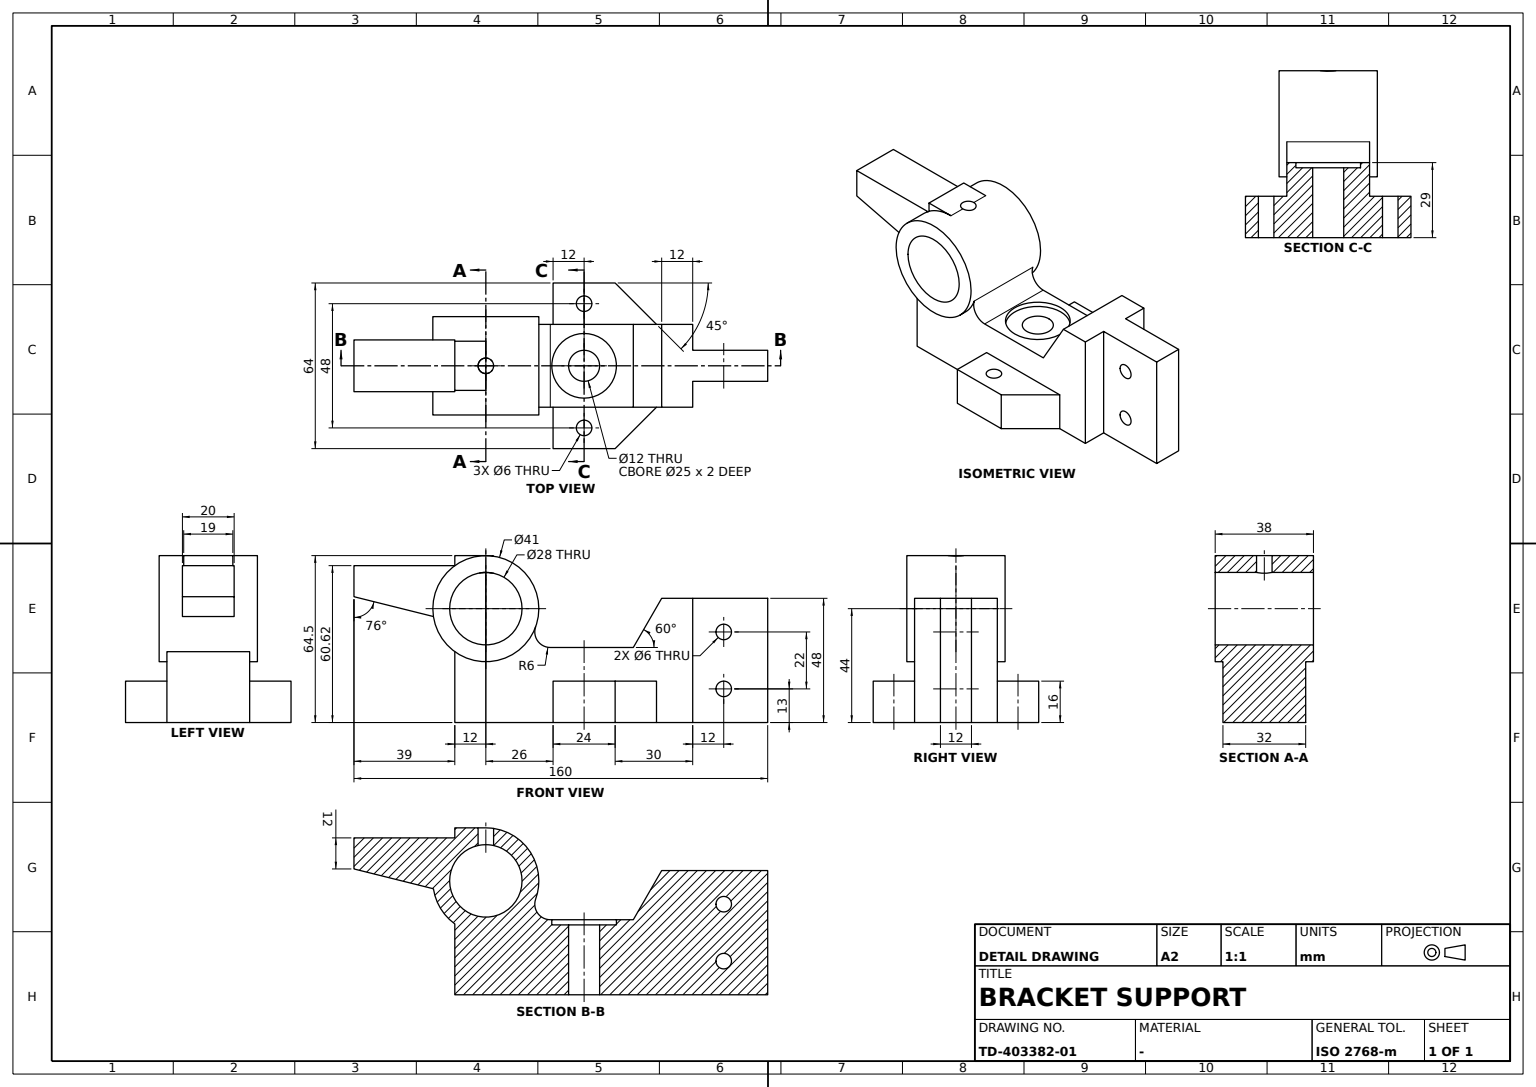
CATIA V5 part; units mm, degrees
sketch "Sketch1" plane through (0, 0, 0) normal (1, 0, 0) x (0, 1, 0)
  circle A0 centre (0, 0) radius 20.5
  dimension "radius A0" = 20.5
extrude "Pad1" add sketch "Sketch1" along normal mid plane 38
sketch "Sketch2" plane through (19, 0, 0) normal (1, 0, 0) x (0, 1, 0)
  circle A0 centre (0, 0) radius 14
  dimension "radius A0" = 14
extrude "Pocket1" cut sketch "Sketch2" against normal through all
sketch "Sketch3" plane through (0, 0, 0) normal (1, 0, 0) x (0, 1, 0)
  point P0 (-12, -44)
  line L0 (-12, -44) -> (109, -44)
  line L1 (24.9249, -15) -> (109, -15)
  point P1 (109, -15)
  line L2 (109, -44) -> (109, -15)
  point P2 (109, -15)
  circle A0 centre (0, 0) radius 20.5 construction
  arc A1 (-12, -16.6208) -> (19.2815, -6.9623) centre (0, 0) ccw
  arc A2 (19.2815, -6.9623) -> (24.9249, -15) centre (24.9249, -9) ccw
  point P3 (19.2815, -6.9623)
  line L3 (-12, -16.6208) -> (-12, -44)
  point P4 (-12, -16.6208)
  dimension "distance P0 x axis" = 44
  dimension "length L0" = 121
  dimension "distance L1 L0" = 29
  dimension "radius A2" = 6
  constraint horizontal L0 x-axis
  constraint horizontal L1 x-axis
  constraint coincidence P2 L1
  constraint coincidence P1 P2
  constraint coincidence A0 P3
  constraint coincidence A0 P4
  constraint vertical L2 y-axis
  constraint vertical L3 y-axis
  constraint tangency A2 A0
  constraint tangency A2 L1
extrude "Pad2" add sketch "Sketch3" along normal mid plane 32
sketch "Sketch4" plane through (0, 0, -15) normal (0, 0, 1) x (1, 0, 0)
  point P0 (11, 94.5)
  line L0 (16, 109) -> (16, 80)
  line L1 (16, 80) -> (6, 80)
  line L2 (6, 80) -> (6, 109)
  line L3 (6, 109) -> (16, 109)
  line L4 (-16, 109) -> (16, 109) construction
  line L5 (16, 109) -> (16, 24.9249) construction
  dimension "distance L2 y axis" = 6
  dimension "length L0" = 29
  constraint vertical L0 y-axis
  constraint vertical L2 y-axis
  constraint horizontal L1 x-axis
  constraint horizontal L3 x-axis
  constraint equidistance L0 L2 P0
  constraint equidistance L1 L3 P0
  constraint coincidence L3 L4
  constraint coincidence L0 L5
extrude "Pocket2" cut sketch "Sketch4" along normal mid plane 100
sketch "Sketch5" plane through (0, 0, 0) normal (1, 0, 0) x (0, 1, 0)
  line L0 (68, 4) -> (109, 4)
  point P0 (109, 4)
  line L1 (109, -44) -> (80, -44) construction
  line L2 (109, -15) -> (109, -44) construction
  line L3 (109, 4) -> (109, -15)
  point P1 (109, -15)
  line L4 (109, -15) -> (80, -15) construction
  line L5 (68, 4) -> (57.0303, -15)
  point P2 (57.0303, -15)
  line L6 (80, -15) -> (80, -44) construction
  line L7 (109, -15) -> (24.9249, -15) construction
  line L8 (57.0303, -15) -> (109, -15)
  dimension "distance L0 L1" = 48
  dimension "length L0" = 41
  dimension "angle L5 L6" = 30
  constraint horizontal L0 x-axis
  constraint horizontal L8 x-axis
  constraint coincidence P0 L2
  constraint coincidence P1 L4
  constraint coincidence P2 L7
  constraint vertical L3 y-axis
extrude "Pad3" add sketch "Sketch5" along normal mid plane 32
sketch "Sketch6" plane through (0, 0, 4) normal (0, 0, 1) x (1, 0, 0)
  point P0 (11, 94.5)
  line L0 (16, 109) -> (16, 80)
  line L1 (16, 80) -> (6, 80)
  line L2 (6, 80) -> (6, 109)
  line L3 (6, 109) -> (16, 109)
  point P1 (16, 109)
  point P2 (16, 80)
  point P3 (6, 80)
  point P4 (6, 109)
  line L4 (16, 109) -> (16, 68) construction
  line L5 (-16, 68) -> (16, 68) construction
  line L6 (-16, 109) -> (16, 109) construction
  point P5 (-11, 94.5)
  point P6 (-16, 109)
  point P7 (-16, 80)
  point P8 (-6, 80)
  point P9 (-6, 109)
  line L7 (-16, 109) -> (-16, 80)
  line L8 (-16, 80) -> (-6, 80)
  line L9 (-6, 80) -> (-6, 109)
  line L10 (-6, 109) -> (-16, 109)
  dimension "distance L2 y axis" = 6
  dimension "distance L5 L1" = 12
  constraint vertical L0 y-axis
  constraint vertical L2 y-axis
  constraint horizontal L1 x-axis
  constraint horizontal L3 x-axis
  constraint equidistance L0 L2 P0
  constraint equidistance L1 L3 P0
  constraint coincidence L0 L4
  constraint coincidence L3 L6
  constraint symmetry P0 P5 y-axis
  constraint symmetry P1 P6 y-axis
  constraint symmetry P2 P7 y-axis
  constraint symmetry P3 P8 y-axis
  constraint symmetry P4 P9 y-axis
  constraint symmetry L0 L7 y-axis
  constraint symmetry L1 L8 y-axis
  constraint symmetry L2 L9 y-axis
  constraint symmetry L3 L10 y-axis
extrude "Pocket3" cut sketch "Sketch6" against normal blind 50
sketch "Sketch7" plane through (0, 0, -44) normal (0, 0, -1) x (1, 0, 0)
  line L0 (-16, -26) -> (-32, -26)
  point P0 (-16, -26)
  line L1 (-16, 12) -> (16, 12) construction
  line L2 (-16, 12) -> (-16, -109) construction
  line L3 (-32, -26) -> (-32, -50)
  point P1 (-32, -50)
  line L4 (-32, -50) -> (-16, -66)
  point P2 (-16, -66)
  line L5 (-16, -26) -> (-16, -66)
  dimension "distance L0 L1" = 38
  dimension "length L3" = 24
  dimension "distance P2 P1 y axis" = 16
  dimension "distance P2 P1 x axis" = 16
  constraint horizontal L0 x-axis
  constraint coincidence P0 L2
  constraint vertical L3 y-axis
  constraint vertical L5 y-axis
extrude "Pad4" add sketch "Sketch7" against normal blind 16
sketch "Sketch8" plane through (0, 0, -44) normal (0, 0, -1) x (1, 0, 0)
  line L0 (16, -26) -> (32, -26)
  point P0 (16, -26)
  line L1 (-16, 12) -> (16, 12) construction
  line L2 (16, 12) -> (16, -109) construction
  line L3 (32, -26) -> (32, -50)
  point P1 (32, -50)
  line L4 (32, -50) -> (16, -66)
  point P2 (16, -66)
  line L5 (16, -26) -> (16, -66)
  dimension "distance L0 L1" = 38
  dimension "length L0" = 16
  dimension "length L3" = 24
  dimension "distance P2 P1 y axis" = 16
  constraint horizontal L0 x-axis
  constraint coincidence P0 L2
  constraint coincidence P2 L2
  constraint vertical L3 y-axis
  constraint vertical L5 y-axis
extrude "Pad5" add sketch "Sketch8" against normal blind 16
sketch "Sketch9" plane through (0, 0, -28) normal (0, 0, 1) x (1, 0, 0)
  circle A0 centre (24, 38) radius 3
  point P0 (24, 38)
  dimension "D1" = 38
  dimension "distance P0 y axis" = 24
  dimension "radius A0" = 3
extrude "Pocket4" cut sketch "Sketch9" against normal blind 16
sketch "Sketch10" plane through (0, 0, -28) normal (0, 0, 1) x (1, 0, 0)
  circle A0 centre (-24, 38) radius 3
  point P0 (-24, 38)
  dimension "distance P0 x axis" = 38
  dimension "distance P0 y axis" = 24
  dimension "radius A0" = 3
extrude "Pocket5" cut sketch "Sketch10" against normal blind 16
sketch "Sketch11" plane through (3.0136, 37.0783, -15) normal (0, 0, 1) x (1, 0, 0)
  point P0 (-3.0136, 0.9217)
  dimension "D1" = 38
hole "Hole1" at (0, 38, -15) direction (0, 0, -1) diameter 12 depth 55 tip angle 120 counterbore diameter 25 counterbore depth 2
sketch "Sketch12" plane through (6, 0, 0) normal (1, 0, 0) x (0, 1, 0)
  circle A0 centre (92, -9) radius 3
  point P0 (92, -9)
  line L0 (109, 4) -> (80, 4) construction
  dimension "distance P0 L0" = 13
  dimension "D2" = 54
  dimension "radius A0" = 3
extrude "Pocket6" cut sketch "Sketch12" against normal blind 16
sketch "Sketch13" plane through (6, 0, 0) normal (1, 0, 0) x (0, 1, 0)
  circle A0 centre (92, -31) radius 3
  point P0 (92, -31)
  line L0 (109, -44) -> (80, -44) construction
  dimension "distance P0 L0" = 13
  dimension "D2" = 54
  dimension "radius A0" = 3
extrude "Pocket7" cut sketch "Sketch13" against normal blind 16
sketch "Sketch14" plane through (0, 0, 0) normal (1, 0, 0) x (0, 1, 0)
  line L0 (0, 20.5) -> (-12, 20.5)
  point P0 (0, 20.5)
  circle A0 centre (0, 0) radius 20.5 construction
  circle A1 centre (0, 0) radius 20.5 construction
  arc A2 (0, 20.5) -> (-12, 16.6208) centre (0, 0) ccw
  line L1 (-12, 20.5) -> (-12, 16.6208)
  point P1 (-12, 16.6208)
  dimension "length L0" = 12
  constraint coincidence P0 y-axis
  constraint coincidence P1 A1
  constraint horizontal L0 x-axis
  constraint tangency L0 A0
  constraint vertical L1 y-axis
extrude "Pad6" add sketch "Sketch14" along normal mid plane 19
sketch "Sketch15" plane through (0, 0, 0) normal (1, 0, 0) x (0, 1, 0)
  line L0 (-12, 16.6208) -> (-51, 16.6208)
  point P0 (-12, 16.6208)
  point P1 (-51, 16.6208)
  circle A0 centre (0, 0) radius 20.5 construction
  line L1 (-12, 20.5) -> (-12, 16.6208) construction
  line L2 (-51, 16.6208) -> (-51, 4.6208)
  line L3 (-51, 4.6208) -> (-20.2733, -3.0403)
  point P2 (-20.2733, -3.0403)
  arc A1 (-12, 16.6208) -> (-20.2733, -3.0403) centre (0, 0) ccw
  dimension "distance P1 y axis" = 51
  dimension "length L2" = 12
  dimension "angle L3 L2" = 104
  constraint horizontal L0 x-axis
  constraint coincidence P0 A0
  constraint coincidence P0 L1
  constraint coincidence P2 A0
  constraint vertical L2 y-axis
extrude "Pad7" add sketch "Sketch15" along normal mid plane 20
sketch "Sketch16" plane through (0, 0, 20.5) normal (0, 0, 1) x (1, 0, 0)
  circle A0 centre (0, 0) radius 3
  dimension "radius A0" = 3
extrude "Pocket8" cut sketch "Sketch16" against normal blind 10
